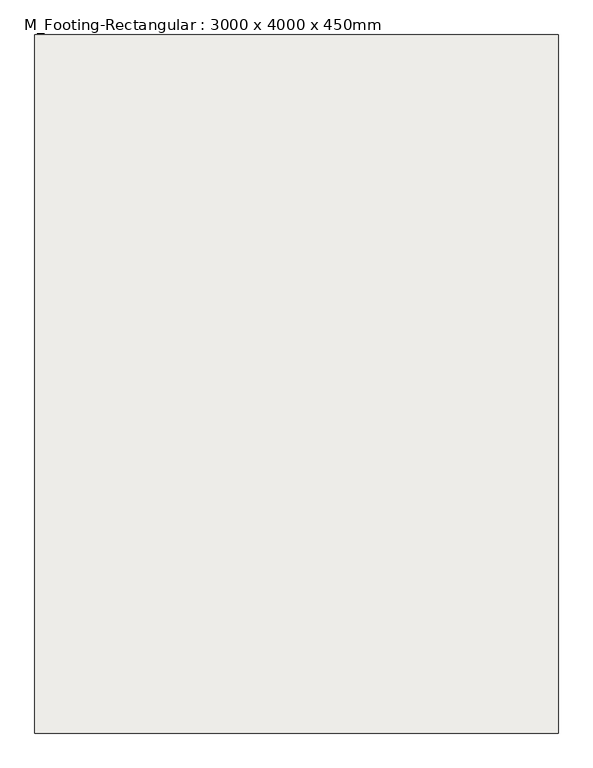
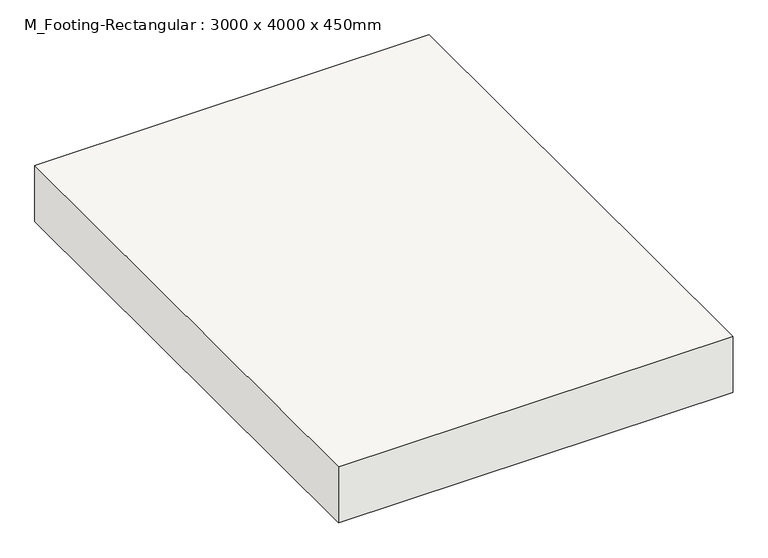
"""IFC4 building model written with IfcOpenShell, lengths in millimetres: slab geometry, M_Footing-Rectangular : 3000 x 4000 x 450mm."""

from ifc_helpers import new_model, si_unit, frame, origin, place, context, project, spatial, polyline, outline, extrude, source, transform, mapped, element, save


def m_footing_rectangular_3000_x_4000_x_450mm_fa7846ad(model_context):
    return source(origin(), model_context, "Body", "SweptSolid", [
        extrude(outline(polyline([(1500.0, 2000.0), (1500.0, -2000.0), (-1500.0, -2000.0), (-1500.0, 2000.0), (1500.0, 2000.0)])), frame((0.0, 0.0, -450.0), z_axis=(0.0, 0.0, 1.0), x_axis=(1.0, 0.0, 0.0)), (0.0, 0.0, 1.0), 450.0),
    ])


if __name__ == "__main__":
    model = new_model("IFC4")
    model_context = context("Model", 3, world=origin())
    ifc_project = project(units=[si_unit("LENGTHUNIT", "METRE", prefix="MILLI")], contexts=[model_context])
    site = spatial("IfcSite", under=ifc_project)
    building = spatial("IfcBuilding", under=site)
    placement = place(None, origin())
    m_footing_rectangular_3000_x_4000_x_450mm_shape = m_footing_rectangular_3000_x_4000_x_450mm_fa7846ad(model_context)
    element("IfcSlab", 1, ObjectType="M_Footing-Rectangular : 3000 x 4000 x 450mm", at=placement, inside=building, context=model_context, shape_type="MappedRepresentation", body=[
        mapped(m_footing_rectangular_3000_x_4000_x_450mm_shape, transform((0.0, 0.0, 0.0), x_axis=(1.0, 0.0, 0.0), y_axis=(0.0, 1.0, 0.0), z_axis=(0.0, 0.0, 1.0))),
    ])
    save(model, "model.ifc")

# Revit data of these elements
# Type "M_Footing-Rectangular : 3000 x 4000 x 450mm"
#   Width = 9' - 10.11024"
#   Length = 13' - 1.48031"
#   Foundation Thickness = 1' - 5.71654"
#   Structural Material [instance default] = Concrete, Cast-in-Place gray
#   Assembly Code = ""
# Element 1 (IfcSlab, "M_Footing-Rectangular : 3000 x 4000 x 450mm")
#   Materials on its faces: "Concrete, Cast-in-Place gray"
# Materials
#   "Concrete, Cast-in-Place gray": class "Concrete", colour RGB 192 192 192, transparency 0, Description = "Cast-in-place concrete", Cost = 0
